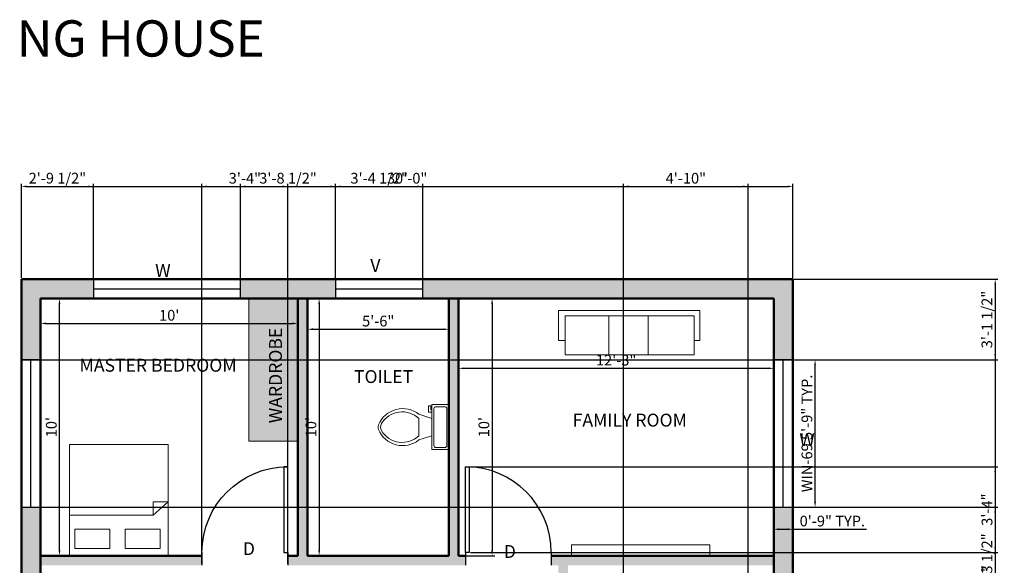
# Model space of a CAD drawing. Units: inches. Extents: x 2064 to 2999, y 1440 to 2089.
# Tile 7 of 7: x 2540 to 2999, y 1835 to 2089. Entities that reach past the tile are written whole.
import ezdxf

# ---------------------------------------------------------------- set-up
doc = ezdxf.new("R2010")
doc.units = ezdxf.units.IN
for name, color, linetype, lineweight in [('A-ANNO-DIMS', 2, 'Continuous', 18), ('A-ANNO-TEXT', 3, 'Continuous', 18), ('A-AREA-IDEN', 7, 'Continuous', 18), ('A-DOOR', 4, 'Continuous', 25), ('A-FLOR-FIXT', 9, 'Continuous', 18), ('A-FURN', 8, 'Continuous', 18), ('A-FURN-PATT', 252, 'Continuous', 13), ('A-GLAZ', 3, 'Continuous', 25), ('A-WALL', 7, 'Continuous', 50), ('A-WALL-PATT', 8, 'Continuous', 13)]:
    doc.layers.add(name, color=color, linetype=linetype, lineweight=lineweight)
doc.styles.get("Standard").update_dxf_attribs({"font": 'arial.ttf'})
doc.dimstyles.new('ISO-25', dxfattribs={"dimtxt": 5, "dimasz": 2.5, "dimexe": 1.25, "dimexo": 0.625, "dimtad": 1, "dimdec": 0, "dimlunit": 4, "dimtxsty": 'Standard', "dimcen": 2.5, "dimadec": 0, "dimazin": 0, "dimtfac": 1, "dimtdec": 0, "dimtmove": 0, "dimatfit": 3, "dimfxl": 1, "dimarcsym": 0})

# ---------------------------------------------------------------- blocks, each defined once
blk = doc.blocks.new('*U2')
for p, q in [((0, 0), (0, -6)), ((40, 0), (40, -6))]:
    blk.add_line(p, q)
blk.add_lwpolyline([(0, 0), (0, 40), (1.75, 40), (1.75, 0)], close=True)
blk.add_arc((0, 0), 40, 0, 90)
blk = doc.blocks.new('*U4')
for p, q in [((9.5, -6), (9.5, -2)), ((-10, -8.5), (-8, -8.5)), ((-10, -9.5), (-10, -8.5)), ((-8, -8.5), (-8, -8)), ((-7, -8), (-7, -9.5)), ((-4, -8), (-6, -14)), ((4, -8), (6, -14)), ((-7, -9.5), (-10, -9.5)), ((4, -14), (-4, -14))]:
    blk.add_line(p, q)
blk.add_lwpolyline([(10.5, -8), (10.5, 0), (-10.5, 0), (-10.5, -8)], close=True)
for points in [[(-9.5, -2), (-9.5, -6)], [(8.5, -1), (-8.5, -1)], [(-8.5, -7), (8.5, -7)]]:
    blk.add_lwpolyline(points)
for centre, radius, start, end in [((-8.62, -1.88), 0.884, 81.8699, 188.1301), ((8.62, -1.88), 0.884, 351.8699, 98.1301), ((-8.62, -6.12), 0.884, 171.8699, 278.1301), ((8.62, -6.12), 0.884, 261.8699, 8.1301), ((3.52, -21.58), 12.17, 141.4691, 247.9714), ((4.2, -21.82), 11.33, 136.3677, 238.9468), ((-3.52, -21.58), 12.17, 292.0284, 38.5307), ((-4.2, -21.82), 11.33, 301.053, 43.6321), ((0, -27.88), 4, 245.7318, 294.2682), ((0, -29), 4, 254.8605, 285.1395)]:
    blk.add_arc(centre, radius, start, end)
blk = doc.blocks.new('*D19')
at = {"layer": 'A-ANNO-DIMS', "color": 0, "lineweight": -2, "transparency": 16777216}
for p, q in [((2549.87, 1958.45), (2549.87, 1946.21)), ((2669.87, 1958.45), (2669.87, 1946.21)), ((2552.37, 1947.46), (2667.37, 1947.46))]:
    blk.add_line(p, q, dxfattribs=at)
at = {"layer": 'A-ANNO-DIMS', "color": 0, "transparency": 16777216}
for points in [[(2552.37, 1947.88), (2552.37, 1947.05), (2549.87, 1947.46)], [(2667.37, 1947.88), (2667.37, 1947.05), (2669.87, 1947.46)]]:
    blk.add_solid(points, dxfattribs=at)
at = {"layer": 'Defpoints', "color": 0, "transparency": 16777216}
for p in [(2549.87, 1959.07), (2669.87, 1959.07), (2669.87, 1947.46)]:
    blk.add_point(p, dxfattribs=at)
at = {"layer": 'A-ANNO-DIMS', "color": 0, "transparency": 16777216, "insert": (2609.87, 1950.64), "char_height": 5, "attachment_point": 5}
blk.add_mtext("10'", dxfattribs=at)
blk = doc.blocks.new('*D20')
at = {"layer": 'A-ANNO-DIMS', "color": 0, "lineweight": -2, "transparency": 16777216}
for p, q in [((2550.5, 1959.07), (2559.93, 1959.07)), ((2558.68, 1841.57), (2558.68, 1956.57)), ((2550.5, 1839.07), (2559.93, 1839.07))]:
    blk.add_line(p, q, dxfattribs=at)
at = {"layer": 'A-ANNO-DIMS', "color": 0, "transparency": 16777216}
for points in [[(2558.26, 1956.57), (2559.09, 1956.57), (2558.68, 1959.07)], [(2558.26, 1841.57), (2559.09, 1841.57), (2558.68, 1839.07)]]:
    blk.add_solid(points, dxfattribs=at)
at = {"layer": 'Defpoints', "color": 0, "transparency": 16777216}
for p in [(2549.87, 1959.07), (2558.68, 1959.07), (2549.87, 1839.07)]:
    blk.add_point(p, dxfattribs=at)
at = {"layer": 'A-ANNO-DIMS', "color": 0, "transparency": 16777216, "insert": (2555.5, 1899.07), "char_height": 5, "attachment_point": 5, "rotation": 90}
blk.add_mtext("10'", dxfattribs=at)
blk = doc.blocks.new('*D21')
at = {"layer": 'A-ANNO-DIMS', "color": 0, "lineweight": -2, "transparency": 16777216}
for p, q in [((2674.37, 1958.45), (2674.37, 1943.51)), ((2740.37, 1958.45), (2740.37, 1943.51)), ((2676.87, 1944.76), (2737.87, 1944.76))]:
    blk.add_line(p, q, dxfattribs=at)
at = {"layer": 'A-ANNO-DIMS', "color": 0, "transparency": 16777216}
for points in [[(2676.87, 1945.17), (2676.87, 1944.34), (2674.37, 1944.76)], [(2737.87, 1945.17), (2737.87, 1944.34), (2740.37, 1944.76)]]:
    blk.add_solid(points, dxfattribs=at)
at = {"layer": 'Defpoints', "color": 0, "transparency": 16777216}
for p in [(2674.37, 1959.07), (2740.37, 1959.07), (2740.37, 1944.76)]:
    blk.add_point(p, dxfattribs=at)
at = {"layer": 'A-ANNO-DIMS', "color": 0, "transparency": 16777216, "insert": (2707.37, 1947.93), "char_height": 5, "attachment_point": 5}
blk.add_mtext('5\'-6"', dxfattribs=at)
blk = doc.blocks.new('*D22')
at = {"layer": 'A-ANNO-DIMS', "color": 0, "lineweight": -2, "transparency": 16777216}
for p, q in [((2675, 1959.07), (2681.07, 1959.07)), ((2679.82, 1956.57), (2679.82, 1841.57)), ((2675, 1839.07), (2681.07, 1839.07))]:
    blk.add_line(p, q, dxfattribs=at)
at = {"layer": 'A-ANNO-DIMS', "color": 0, "transparency": 16777216}
for points in [[(2679.4, 1956.57), (2680.24, 1956.57), (2679.82, 1959.07)], [(2679.4, 1841.57), (2680.24, 1841.57), (2679.82, 1839.07)]]:
    blk.add_solid(points, dxfattribs=at)
at = {"layer": 'Defpoints', "color": 0, "transparency": 16777216}
for p in [(2674.37, 1959.07), (2674.37, 1839.07), (2679.82, 1839.07)]:
    blk.add_point(p, dxfattribs=at)
at = {"layer": 'A-ANNO-DIMS', "color": 0, "transparency": 16777216, "insert": (2676.64, 1899.07), "char_height": 5, "attachment_point": 5, "rotation": 90}
blk.add_mtext("10'", dxfattribs=at)
blk = doc.blocks.new('*D23')
at = {"layer": 'A-ANNO-DIMS', "color": 0, "lineweight": -2, "transparency": 16777216}
for p, q in [((2744.87, 1958.45), (2744.87, 1925.27)), ((2891.87, 1958.45), (2891.87, 1925.27)), ((2747.37, 1926.52), (2889.37, 1926.52))]:
    blk.add_line(p, q, dxfattribs=at)
at = {"layer": 'A-ANNO-DIMS', "color": 0, "transparency": 16777216}
for points in [[(2747.37, 1926.94), (2747.37, 1926.11), (2744.87, 1926.52)], [(2889.37, 1926.94), (2889.37, 1926.11), (2891.87, 1926.52)]]:
    blk.add_solid(points, dxfattribs=at)
at = {"layer": 'Defpoints', "color": 0, "transparency": 16777216}
for p in [(2744.87, 1959.07), (2891.87, 1959.07), (2891.87, 1926.52)]:
    blk.add_point(p, dxfattribs=at)
at = {"layer": 'A-ANNO-DIMS', "color": 0, "transparency": 16777216, "insert": (2818.37, 1929.7), "char_height": 5, "attachment_point": 5}
blk.add_mtext('12\'-3"', dxfattribs=at)
blk = doc.blocks.new('*D24')
at = {"layer": 'A-ANNO-DIMS', "color": 0, "lineweight": -2, "transparency": 16777216}
for p, q in [((2745.5, 1959.07), (2761.75, 1959.07)), ((2760.5, 1956.57), (2760.5, 1841.57)), ((2745.5, 1839.07), (2761.75, 1839.07))]:
    blk.add_line(p, q, dxfattribs=at)
at = {"layer": 'A-ANNO-DIMS', "color": 0, "transparency": 16777216}
for points in [[(2760.08, 1956.57), (2760.91, 1956.57), (2760.5, 1959.07)], [(2760.08, 1841.57), (2760.91, 1841.57), (2760.5, 1839.07)]]:
    blk.add_solid(points, dxfattribs=at)
at = {"layer": 'Defpoints', "color": 0, "transparency": 16777216}
for p in [(2744.87, 1959.07), (2744.87, 1839.07), (2760.5, 1839.07)]:
    blk.add_point(p, dxfattribs=at)
at = {"layer": 'A-ANNO-DIMS', "color": 0, "transparency": 16777216, "insert": (2757.32, 1899.07), "char_height": 5, "attachment_point": 5, "rotation": 90}
blk.add_mtext("10'", dxfattribs=at)
blk = doc.blocks.new('SOFA-3')
for p, q in [((0, 0), (0, 65.92)), ((0, 65.92), (14.01, 65.92)), ((14.01, 65.92), (14.01, 63.25)), ((20.61, 41.74), (2.39, 41.74)), ((20.61, 23.49), (2.39, 23.49)), ((14.01, 3.1), (14.01, 0)), ((14.01, 0), (0, 0))]:
    blk.add_line(p, q)
blk.add_lwpolyline([(2.39, 3.1), (20.61, 3.1), (20.61, 63.25), (2.39, 63.25)], close=True)
blk = doc.blocks.new('WIN-69')
blk.add_line((4.5, 0), (4.5, 68.8))
blk.add_lwpolyline([(0, 0), (9, 0), (9, 68.8), (0, 68.8)], close=True)
blk = doc.blocks.new('*D61')
at = {"layer": 'A-ANNO-DIMS', "color": 0, "lineweight": -2, "transparency": 16777216}
for p, q in [((2901.5, 1930.52), (2912.44, 1930.52)), ((2911.19, 1864.22), (2911.19, 1928.02)), ((2901.5, 1861.72), (2912.44, 1861.72))]:
    blk.add_line(p, q, dxfattribs=at)
at = {"layer": 'A-ANNO-DIMS', "color": 0, "transparency": 16777216}
for points in [[(2910.78, 1928.02), (2911.61, 1928.02), (2911.19, 1930.52)], [(2910.78, 1864.22), (2911.61, 1864.22), (2911.19, 1861.72)]]:
    blk.add_solid(points, dxfattribs=at)
at = {"layer": 'Defpoints', "color": 0, "transparency": 16777216}
for p in [(2900.87, 1930.52), (2911.19, 1930.52), (2900.87, 1861.72)]:
    blk.add_point(p, dxfattribs=at)
at = {"layer": 'A-ANNO-DIMS', "color": 0, "transparency": 16777216, "insert": (2908.02, 1896.12), "char_height": 5, "attachment_point": 5, "rotation": 90}
blk.add_mtext('WIN-69 5\'-9" TYP.', dxfattribs=at)
blk = doc.blocks.new('*D62')
at = {"layer": 'A-ANNO-DIMS', "color": 0, "lineweight": -2, "transparency": 16777216}
for p, q in [((2891.87, 1861.1), (2891.87, 1850.15)), ((2900.87, 1861.1), (2900.87, 1850.15)), ((2894.37, 1851.4), (2898.37, 1851.4)), ((2900.87, 1851.4), (2935.1, 1851.4))]:
    blk.add_line(p, q, dxfattribs=at)
at = {"layer": 'A-ANNO-DIMS', "color": 0, "transparency": 16777216}
for points in [[(2894.37, 1851.82), (2894.37, 1850.99), (2891.87, 1851.4)], [(2898.37, 1851.82), (2898.37, 1850.99), (2900.87, 1851.4)]]:
    blk.add_solid(points, dxfattribs=at)
at = {"layer": 'Defpoints', "color": 0, "transparency": 16777216}
for p in [(2891.87, 1861.72), (2900.87, 1861.72), (2900.87, 1851.4)]:
    blk.add_point(p, dxfattribs=at)
at = {"layer": 'A-ANNO-DIMS', "color": 0, "transparency": 16777216, "insert": (2919.24, 1854.58), "char_height": 5, "attachment_point": 5}
blk.add_mtext('0\'-9" TYP.', dxfattribs=at)
blk = doc.blocks.new('*D82')
at = {"layer": 'A-ANNO-DIMS', "color": 0, "lineweight": -2, "transparency": 16777216}
for p, q in [((2540.87, 1968.7), (2540.87, 2012.67)), ((2900.87, 1968.7), (2900.87, 2012.67)), ((2543.37, 2011.42), (2898.37, 2011.42))]:
    blk.add_line(p, q, dxfattribs=at)
at = {"layer": 'A-ANNO-DIMS', "color": 0, "transparency": 16777216}
for points in [[(2543.37, 2011.84), (2543.37, 2011), (2540.87, 2011.42)], [(2898.37, 2011.84), (2898.37, 2011), (2900.87, 2011.42)]]:
    blk.add_solid(points, dxfattribs=at)
at = {"layer": 'Defpoints', "color": 0, "transparency": 16777216}
for p in [(2900.87, 2011.42), (2540.87, 1968.07), (2900.87, 1968.07)]:
    blk.add_point(p, dxfattribs=at)
at = {"layer": 'A-ANNO-DIMS', "color": 0, "transparency": 16777216, "insert": (2720.87, 2014.6), "char_height": 5, "attachment_point": 5}
blk.add_mtext('30\'-0"', dxfattribs=at)
blk = doc.blocks.new('*D83')
at = {"layer": 'A-ANNO-DIMS', "color": 0, "lineweight": -2, "transparency": 16777216}
for p, q in [((2901.5, 1968.07), (2996.47, 1968.07)), ((2995.22, 1965.57), (2995.22, 1490.57)), ((2901.5, 1488.07), (2996.47, 1488.07))]:
    blk.add_line(p, q, dxfattribs=at)
at = {"layer": 'A-ANNO-DIMS', "color": 0, "transparency": 16777216}
for points in [[(2994.81, 1965.57), (2995.64, 1965.57), (2995.22, 1968.07)], [(2994.81, 1490.57), (2995.64, 1490.57), (2995.22, 1488.07)]]:
    blk.add_solid(points, dxfattribs=at)
at = {"layer": 'Defpoints', "color": 0, "transparency": 16777216}
for p in [(2900.87, 1968.07), (2900.87, 1488.07), (2995.22, 1488.07)]:
    blk.add_point(p, dxfattribs=at)
at = {"layer": 'A-ANNO-DIMS', "color": 0, "transparency": 16777216, "insert": (2992.05, 1728.07), "char_height": 5, "attachment_point": 5, "rotation": 90}
blk.add_mtext('40\'-0"', dxfattribs=at)
blk = doc.blocks.new('*D84')
at = {"layer": 'A-ANNO-DIMS', "color": 0, "lineweight": -2, "transparency": 16777216}
for p, q in [((2540.87, 1968.7), (2540.87, 2012.67)), ((2574.52, 1968.7), (2574.52, 2012.67)), ((2543.37, 2011.42), (2572.02, 2011.42))]:
    blk.add_line(p, q, dxfattribs=at)
at = {"layer": 'A-ANNO-DIMS', "color": 0, "transparency": 16777216}
for points in [[(2543.37, 2011.84), (2543.37, 2011), (2540.87, 2011.42)], [(2572.02, 2011.84), (2572.02, 2011), (2574.52, 2011.42)]]:
    blk.add_solid(points, dxfattribs=at)
at = {"layer": 'Defpoints', "color": 0, "transparency": 16777216}
for p in [(2574.52, 2011.42), (2540.87, 1968.07), (2574.52, 1968.07)]:
    blk.add_point(p, dxfattribs=at)
at = {"layer": 'A-ANNO-DIMS', "color": 0, "transparency": 16777216, "insert": (2557.7, 2014.63), "char_height": 5, "attachment_point": 5}
blk.add_mtext('2\'-9 1/2"', dxfattribs=at)
blk = doc.blocks.new('*D85')
at = {"layer": 'A-ANNO-DIMS', "color": 0, "lineweight": -2, "transparency": 16777216}
for p, q in [((2643.06, 1968.7), (2643.06, 2012.67)), ((2687.51, 1968.7), (2687.51, 2012.67)), ((2645.56, 2011.42), (2685.01, 2011.42))]:
    blk.add_line(p, q, dxfattribs=at)
at = {"layer": 'A-ANNO-DIMS', "color": 0, "transparency": 16777216}
for points in [[(2645.56, 2011.84), (2645.56, 2011), (2643.06, 2011.42)], [(2685.01, 2011.84), (2685.01, 2011), (2687.51, 2011.42)]]:
    blk.add_solid(points, dxfattribs=at)
at = {"layer": 'Defpoints', "color": 0, "transparency": 16777216}
for p in [(2687.51, 2011.42), (2643.06, 1968.07), (2687.51, 1968.07)]:
    blk.add_point(p, dxfattribs=at)
at = {"layer": 'A-ANNO-DIMS', "color": 0, "transparency": 16777216, "insert": (2665.29, 2014.63), "char_height": 5, "attachment_point": 5}
blk.add_mtext('3\'-8 1/2"', dxfattribs=at)
blk = doc.blocks.new('*D86')
at = {"layer": 'A-ANNO-DIMS', "color": 0, "lineweight": -2, "transparency": 16777216}
for p, q in [((2687.51, 1968.7), (2687.51, 2012.67)), ((2728.11, 1968.7), (2728.11, 2012.67)), ((2690.01, 2011.42), (2725.61, 2011.42))]:
    blk.add_line(p, q, dxfattribs=at)
at = {"layer": 'A-ANNO-DIMS', "color": 0, "transparency": 16777216}
for points in [[(2690.01, 2011.84), (2690.01, 2011), (2687.51, 2011.42)], [(2725.61, 2011.84), (2725.61, 2011), (2728.11, 2011.42)]]:
    blk.add_solid(points, dxfattribs=at)
at = {"layer": 'Defpoints', "color": 0, "transparency": 16777216}
for p in [(2728.11, 2011.42), (2687.51, 1968.07), (2728.11, 1968.07)]:
    blk.add_point(p, dxfattribs=at)
at = {"layer": 'A-ANNO-DIMS', "color": 0, "transparency": 16777216, "insert": (2707.81, 2014.63), "char_height": 5, "attachment_point": 5}
blk.add_mtext('3\'-4 1/2"', dxfattribs=at)
blk = doc.blocks.new('*D87')
at = {"layer": 'A-ANNO-DIMS', "color": 0, "lineweight": -2, "transparency": 16777216}
for p, q in [((2901.5, 1968.07), (2996.47, 1968.07)), ((2995.22, 1965.57), (2995.22, 1933.02)), ((2901.5, 1930.52), (2996.47, 1930.52))]:
    blk.add_line(p, q, dxfattribs=at)
at = {"layer": 'A-ANNO-DIMS', "color": 0, "transparency": 16777216}
for points in [[(2994.81, 1965.57), (2995.64, 1965.57), (2995.22, 1968.07)], [(2994.81, 1933.02), (2995.64, 1933.02), (2995.22, 1930.52)]]:
    blk.add_solid(points, dxfattribs=at)
at = {"layer": 'Defpoints', "color": 0, "transparency": 16777216}
for p in [(2900.87, 1968.07), (2900.87, 1930.52), (2995.22, 1930.52)]:
    blk.add_point(p, dxfattribs=at)
at = {"layer": 'A-ANNO-DIMS', "color": 0, "transparency": 16777216, "insert": (2992.01, 1949.3), "char_height": 5, "attachment_point": 5, "rotation": 90}
blk.add_mtext('3\'-1 1/2"', dxfattribs=at)
blk = doc.blocks.new('*D88')
at = {"layer": 'A-ANNO-DIMS', "color": 0, "lineweight": -2, "transparency": 16777216}
for p, q in [((2901.5, 1861.72), (2996.47, 1861.72)), ((2995.22, 1859.22), (2995.22, 1812.91)), ((2901.5, 1810.41), (2996.47, 1810.41))]:
    blk.add_line(p, q, dxfattribs=at)
at = {"layer": 'A-ANNO-DIMS', "color": 0, "transparency": 16777216}
for points in [[(2994.81, 1859.22), (2995.64, 1859.22), (2995.22, 1861.72)], [(2994.81, 1812.91), (2995.64, 1812.91), (2995.22, 1810.41)]]:
    blk.add_solid(points, dxfattribs=at)
at = {"layer": 'Defpoints', "color": 0, "transparency": 16777216}
for p in [(2900.87, 1861.72), (2900.87, 1810.41), (2995.22, 1810.41)]:
    blk.add_point(p, dxfattribs=at)
at = {"layer": 'A-ANNO-DIMS', "color": 0, "transparency": 16777216, "insert": (2992.01, 1836.07), "char_height": 5, "attachment_point": 5, "rotation": 90}
blk.add_mtext('4\'-3 1/2"', dxfattribs=at)
blk = doc.blocks.new('*D91')
at = {"layer": 'A-ANNO-DIMS', "color": 0, "lineweight": -2, "transparency": 16777216}
for p, q in [((2541.5, 1968.07), (2996.47, 1968.07)), ((2995.22, 1965.57), (2995.22, 1933.02)), ((2541.5, 1930.52), (2996.47, 1930.52))]:
    blk.add_line(p, q, dxfattribs=at)
at = {"layer": 'A-ANNO-DIMS', "color": 0, "transparency": 16777216}
for points in [[(2994.81, 1965.57), (2995.64, 1965.57), (2995.22, 1968.07)], [(2994.81, 1933.02), (2995.64, 1933.02), (2995.22, 1930.52)]]:
    blk.add_solid(points, dxfattribs=at)
at = {"layer": 'Defpoints', "color": 0, "transparency": 16777216}
for p in [(2540.87, 1968.07), (2540.87, 1930.52), (2995.22, 1930.52)]:
    blk.add_point(p, dxfattribs=at)
at = {"layer": 'A-ANNO-DIMS', "color": 0, "transparency": 16777216, "insert": (2992.01, 1949.3), "char_height": 5, "attachment_point": 5, "rotation": 90}
blk.add_mtext('3\'-1 1/2"', dxfattribs=at)
blk = doc.blocks.new('*D92')
at = {"layer": 'A-ANNO-DIMS', "color": 0, "lineweight": -2, "transparency": 16777216}
for p, q in [((2541.5, 1861.72), (2996.47, 1861.72)), ((2995.22, 1859.22), (2995.22, 1795.07)), ((2541.5, 1792.57), (2996.47, 1792.57))]:
    blk.add_line(p, q, dxfattribs=at)
at = {"layer": 'A-ANNO-DIMS', "color": 0, "transparency": 16777216}
for points in [[(2994.81, 1859.22), (2995.64, 1859.22), (2995.22, 1861.72)], [(2994.81, 1795.07), (2995.64, 1795.07), (2995.22, 1792.57)]]:
    blk.add_solid(points, dxfattribs=at)
at = {"layer": 'Defpoints', "color": 0, "transparency": 16777216}
for p in [(2540.87, 1861.72), (2540.87, 1792.57), (2995.22, 1792.57)]:
    blk.add_point(p, dxfattribs=at)
at = {"layer": 'A-ANNO-DIMS', "color": 0, "transparency": 16777216, "insert": (2992.05, 1827.15), "char_height": 5, "attachment_point": 5, "rotation": 90}
blk.add_mtext('5\'-9"', dxfattribs=at)
blk = doc.blocks.new('*D104')
at = {"layer": 'A-ANNO-DIMS', "color": 0, "lineweight": -2, "transparency": 16777216}
for p, q in [((2821.8, 1758.7), (2821.8, 2012.67)), ((2879.97, 1758.7), (2879.97, 2012.67)), ((2824.3, 2011.42), (2877.47, 2011.42))]:
    blk.add_line(p, q, dxfattribs=at)
at = {"layer": 'A-ANNO-DIMS', "color": 0, "transparency": 16777216}
for points in [[(2824.3, 2011.84), (2824.3, 2011), (2821.8, 2011.42)], [(2877.47, 2011.84), (2877.47, 2011), (2879.97, 2011.42)]]:
    blk.add_solid(points, dxfattribs=at)
at = {"layer": 'Defpoints', "color": 0, "transparency": 16777216}
for p in [(2879.97, 2011.42), (2821.8, 1758.07), (2879.97, 1758.07)]:
    blk.add_point(p, dxfattribs=at)
at = {"layer": 'A-ANNO-DIMS', "color": 0, "transparency": 16777216, "insert": (2850.89, 2014.6), "char_height": 5, "attachment_point": 5}
blk.add_mtext('4\'-10"', dxfattribs=at)
blk = doc.blocks.new('*D115')
at = {"layer": 'A-ANNO-DIMS', "color": 0, "lineweight": -2, "transparency": 16777216}
for p, q in [((2625.15, 1835.2), (2625.15, 2012.67)), ((2665.15, 1835.2), (2665.15, 2012.67)), ((2627.65, 2011.42), (2662.65, 2011.42))]:
    blk.add_line(p, q, dxfattribs=at)
at = {"layer": 'A-ANNO-DIMS', "color": 0, "transparency": 16777216}
for points in [[(2627.65, 2011.84), (2627.65, 2011), (2625.15, 2011.42)], [(2662.65, 2011.84), (2662.65, 2011), (2665.15, 2011.42)]]:
    blk.add_solid(points, dxfattribs=at)
at = {"layer": 'Defpoints', "color": 0, "transparency": 16777216}
for p in [(2665.15, 2011.42), (2625.15, 1834.57), (2665.15, 1834.57)]:
    blk.add_point(p, dxfattribs=at)
at = {"layer": 'A-ANNO-DIMS', "color": 0, "transparency": 16777216, "insert": (2645.15, 2014.6), "char_height": 5, "attachment_point": 5}
blk.add_mtext('3\'-4"', dxfattribs=at)
blk = doc.blocks.new('*D116')
at = {"layer": 'A-ANNO-DIMS', "color": 0, "lineweight": -2, "transparency": 16777216}
for p, q in [((2750.49, 1880.57), (2996.47, 1880.57)), ((2995.22, 1878.07), (2995.22, 1843.07)), ((2750.49, 1840.57), (2996.47, 1840.57))]:
    blk.add_line(p, q, dxfattribs=at)
at = {"layer": 'A-ANNO-DIMS', "color": 0, "transparency": 16777216}
for points in [[(2994.81, 1878.07), (2995.64, 1878.07), (2995.22, 1880.57)], [(2994.81, 1843.07), (2995.64, 1843.07), (2995.22, 1840.57)]]:
    blk.add_solid(points, dxfattribs=at)
at = {"layer": 'Defpoints', "color": 0, "transparency": 16777216}
for p in [(2749.86, 1880.57), (2749.86, 1840.57), (2995.22, 1840.57)]:
    blk.add_point(p, dxfattribs=at)
at = {"layer": 'A-ANNO-DIMS', "color": 0, "transparency": 16777216, "insert": (2992.05, 1860.57), "char_height": 5, "attachment_point": 5, "rotation": 90}
blk.add_mtext('3\'-4"', dxfattribs=at)

msp = doc.modelspace()

# ---------------------------------------------------------------- hatches: boundary and pattern name
at = {"layer": 'A-FURN-PATT'}
h = msp.add_hatch(color=256, dxfattribs=at)
h.dxf.hatch_style = 1
h.paths.add_polyline_path([(2211.98, 1959.07), (2126.82, 1959.07), (2126.82, 1938.57), (2211.98, 1938.57)])
h.paths.add_polyline_path([(2669.87, 1959.07), (2646.96, 1959.07), (2646.96, 1892.49), (2669.87, 1892.49)])
h.paths.add_polyline_path([(2468.82, 1668.53), (2348.82, 1668.53), (2348.82, 1638.07), (2468.82, 1638.07)])
h.paths.add_polyline_path([(2891.87, 1667.99), (2780.13, 1667.99), (2780.13, 1638.07), (2891.87, 1638.07)])
h.paths.add_polyline_path([(2854.27, 1658.75), (2854.27, 1650.97), (2859.31, 1650.97), (2859.31, 1658.75), (2862.16, 1658.75), (2862.16, 1650.97), (2867.47, 1650.97), (2867.47, 1658.75), (2870.33, 1658.75), (2870.33, 1650.97), (2879.45, 1650.97), (2879.45, 1658.75), (2882.31, 1658.75), (2882.31, 1643.24), (2879.45, 1643.24), (2879.45, 1650.97), (2870.33, 1650.97), (2870.33, 1643.24), (2867.47, 1643.24), (2867.47, 1650.97), (2862.16, 1650.97), (2862.16, 1643.24), (2859.31, 1643.24), (2859.31, 1650.97), (2854.27, 1650.97), (2854.27, 1643.24), (2851.41, 1643.24), (2851.41, 1650.97), (2845.97, 1650.97), (2845.97, 1643.24), (2843.11, 1643.24), (2843.11, 1650.97), (2839.98, 1650.97), (2839.98, 1643.24), (2837.12, 1643.24), (2837.12, 1650.97), (2831.27, 1650.97), (2831.27, 1643.24), (2828.41, 1643.24), (2828.41, 1650.97), (2823.78, 1650.97), (2823.78, 1643.24), (2820.92, 1643.24), (2820.92, 1650.97), (2816.56, 1650.97), (2816.56, 1641.66), (2813.71, 1641.66), (2813.71, 1650.97), (2808.81, 1650.97), (2808.81, 1641.66), (2805.95, 1641.66), (2805.95, 1650.97), (2801.73, 1650.97), (2801.73, 1641.66), (2798.87, 1641.66), (2798.87, 1650.97), (2794.92, 1650.97), (2794.92, 1643.24), (2792.06, 1643.24), (2792.06, 1658.75), (2794.92, 1658.75), (2794.92, 1650.97), (2798.87, 1650.97), (2798.87, 1657.16), (2801.73, 1657.16), (2801.73, 1650.97), (2805.95, 1650.97), (2805.95, 1657.16), (2808.81, 1657.16), (2808.81, 1650.97), (2813.71, 1650.97), (2813.71, 1657.16), (2816.56, 1657.16), (2816.56, 1650.97), (2820.92, 1650.97), (2820.92, 1658.75), (2823.78, 1658.75), (2823.78, 1650.97), (2828.41, 1650.97), (2828.41, 1658.75), (2831.27, 1658.75), (2831.27, 1650.97), (2837.12, 1650.97), (2837.12, 1658.75), (2839.98, 1658.75), (2839.98, 1650.97), (2843.11, 1650.97), (2843.11, 1658.75), (2845.97, 1658.75), (2845.97, 1650.97), (2851.41, 1650.97), (2851.41, 1658.75)], flags=16)
h.paths.add_polyline_path([(2665.84, 1899.31), (2665.84, 1951.8), (2653.45, 1951.8), (2653.45, 1899.31)], flags=24)
h.paths.add_polyline_path([(2565.91, 1921.55), (2649.69, 1921.55), (2649.69, 1933.95), (2565.91, 1933.95)], flags=9)
h.paths.add_polyline_path([(2402.8, 1649), (2414.4, 1649), (2414.4, 1659.3), (2402.8, 1659.3)], flags=24)
at = {"layer": 'A-WALL-PATT'}
h = msp.add_hatch(color=256, dxfattribs=at)
h.dxf.hatch_style = 1
h.paths.add_polyline_path([(2574.52, 1968.07), (2540.87, 1968.07), (2540.87, 1930.52), (2549.87, 1930.52), (2549.87, 1959.07), (2574.52, 1959.07)])
h.paths.add_polyline_path([(2687.51, 1968.07), (2643.06, 1968.07), (2643.06, 1959.07), (2669.87, 1959.07), (2687.51, 1959.07)])
h.paths.add_polyline_path([(2900.87, 1968.07), (2728.11, 1968.07), (2728.11, 1959.07), (2740.37, 1959.07), (2891.87, 1959.07), (2891.87, 1930.52), (2900.87, 1930.52)])
h.paths.add_polyline_path([(2744.87, 1959.07), (2740.37, 1959.07), (2740.37, 1839.07), (2674.37, 1839.07), (2674.37, 1959.07), (2669.87, 1959.07), (2669.87, 1892.49), (2669.87, 1839.07), (2665.15, 1839.07), (2665.15, 1834.57), (2674.37, 1834.57), (2744.87, 1834.57), (2748.11, 1834.57), (2748.11, 1839.07), (2744.87, 1839.07)])
h.paths.add_polyline_path([(2549.87, 1834.57), (2549.87, 1861.72), (2540.87, 1861.72), (2540.87, 1792.57), (2549.87, 1792.57)])
h.paths.add_polyline_path([(2625.15, 1839.07), (2549.87, 1839.07), (2549.87, 1834.57), (2625.15, 1834.57)])
h.paths.add_polyline_path([(2900.87, 1861.72), (2891.87, 1861.72), (2891.87, 1810.41), (2900.87, 1810.41)])
h.paths.add_polyline_path([(2891.87, 1839.07), (2788.11, 1839.07), (2788.11, 1834.57), (2891.87, 1834.57)])
h.paths.add_polyline_path([(2549.87, 1745.09), (2540.87, 1745.09), (2540.87, 1697.07), (2549.87, 1697.07)])
h.paths.add_polyline_path([(2549.87, 1619.25), (2540.87, 1619.25), (2540.87, 1612.26), (2549.87, 1612.26)], flags=17)
h.paths.add_polyline_path([(2549.87, 1516.02), (2540.87, 1516.02), (2540.87, 1488.07), (2900.87, 1488.07), (2900.87, 1682.51), (2891.87, 1682.51), (2891.87, 1497.07), (2549.87, 1497.07)])
h.paths.add_polyline_path([(2771.87, 1575.08), (2767.37, 1575.08), (2767.37, 1497.07), (2771.87, 1497.07)], flags=17)
h.paths.add_polyline_path([(2771.87, 1708.85), (2767.37, 1708.85), (2767.37, 1633.57), (2771.87, 1633.57), (2771.87, 1638.07)])
h.paths.add_polyline_path([(2891.87, 1638.07), (2780.13, 1638.07), (2771.87, 1638.07), (2771.87, 1633.57), (2891.87, 1633.57)], flags=17)
h.paths.add_polyline_path([(2771.87, 1633.57), (2767.37, 1633.57), (2767.37, 1615.08), (2771.87, 1615.08)], flags=17)
h.paths.add_polyline_path([(2900.87, 1784.26), (2891.87, 1784.26), (2891.87, 1751.31), (2900.87, 1751.31)])
h.paths.add_polyline_path([(2795.87, 1834.57), (2791.37, 1834.57), (2791.37, 1830.13), (2795.87, 1830.13)])
h.paths.add_polyline_path([(2805.14, 1771.92), (2830.56, 1771.92), (2830.56, 1784.32), (2805.14, 1784.32)], flags=9)
h.paths.add_polyline_path([(2805.18, 1686.98), (2865.14, 1686.98), (2865.14, 1699.38), (2805.18, 1699.38)], flags=9)
h.paths.add_polyline_path([(2801, 1552.43), (2850.22, 1552.43), (2850.22, 1564.83), (2801, 1564.83)], flags=25)
h.paths.add_polyline_path([(2645.3, 1586.75), (2705.73, 1586.75), (2705.73, 1599.14), (2645.3, 1599.14)], flags=25)
h.paths.add_polyline_path([(2670.49, 1736.4), (2713.67, 1736.4), (2713.67, 1748.79), (2670.49, 1748.79)], flags=9)
h.paths.add_polyline_path([(2795.9, 1895.95), (2857.73, 1895.95), (2857.73, 1908.34), (2795.9, 1908.34)], flags=9)
h.paths.add_polyline_path([(2565.91, 1921.55), (2649.69, 1921.55), (2649.69, 1933.95), (2565.91, 1933.95)], flags=9)

# ---------------------------------------------------------------- linework, layer by layer
at = {"layer": 'A-FURN'}
for p, q in [((2602.33, 1858.02), (2602.33, 1864.23)), ((2602.33, 1864.23), (2609.36, 1864.23)), ((2609.36, 1864.23), (2602.33, 1858.02)), ((2563.4, 1858.02), (2602.33, 1858.02))]:
    msp.add_line(p, q, dxfattribs=at)
for points in [[(2669.87, 1959.07), (2646.96, 1959.07), (2646.96, 1892.49), (2669.87, 1892.49)], [(2563.4, 1839.07), (2609.36, 1839.07), (2609.36, 1891.01), (2563.4, 1891.01)], [(2565.89, 1842.42), (2582.11, 1842.42), (2582.11, 1851.45), (2565.89, 1851.45)], [(2589.38, 1842.42), (2605.6, 1842.42), (2605.6, 1851.45), (2589.38, 1851.45)], [(2797.55, 1839.07), (2862.05, 1839.07), (2862.05, 1844.06), (2797.55, 1844.06)]]:
    msp.add_lwpolyline(points, close=True, dxfattribs=at)
at = {"layer": 'A-GLAZ'}
for p, q in [((2574.52, 1963.57), (2643.06, 1963.57)), ((2687.51, 1963.57), (2728.11, 1963.57))]:
    msp.add_line(p, q, dxfattribs=at)
for points in [[(2574.52, 1959.07), (2643.06, 1959.07), (2643.06, 1968.07), (2574.52, 1968.07)], [(2687.51, 1959.07), (2728.11, 1959.07), (2728.11, 1968.07), (2687.51, 1968.07)]]:
    msp.add_lwpolyline(points, close=True, dxfattribs=at)
at = {"layer": 'A-WALL'}
for p, q in [((2540.87, 1968.07), (2900.87, 1968.07)), ((2540.87, 1488.07), (2540.87, 1968.07)), ((2900.87, 1968.07), (2900.87, 1488.07)), ((2549.87, 1959.07), (2891.87, 1959.07)), ((2549.87, 1497.07), (2549.87, 1959.07)), ((2549.87, 1959.07), (2669.87, 1959.07)), ((2669.87, 1959.07), (2669.87, 1839.07)), ((2674.37, 1959.07), (2674.37, 1839.07)), ((2674.37, 1959.07), (2740.37, 1959.07)), ((2740.37, 1959.07), (2740.37, 1839.07)), ((2744.87, 1959.07), (2744.87, 1839.07)), ((2891.87, 1959.07), (2891.87, 1497.07)), ((2625.15, 1839.07), (2549.87, 1839.07)), ((2669.87, 1839.07), (2665.15, 1839.07)), ((2740.37, 1839.07), (2674.37, 1839.07)), ((2744.87, 1839.07), (2748.11, 1839.07)), ((2788.11, 1839.07), (2891.87, 1839.07))]:
    msp.add_line(p, q, dxfattribs=at)

# ---------------------------------------------------------------- block references
at = {"layer": 'A-DOOR', "xscale": -1}
msp.add_blockref('*U2', (2665.15, 1840.57), dxfattribs=at)
at = {"layer": 'A-DOOR'}
msp.add_blockref('*U2', (2748.11, 1840.57), dxfattribs=at)
at = {"layer": 'A-FLOR-FIXT', "rotation": 270}
msp.add_blockref('*U4', (2740.37, 1899.07), dxfattribs=at)
at = {"layer": 'A-FURN', "rotation": 269.9999999999988}
msp.add_blockref('SOFA-3', (2791.5, 1953.45), dxfattribs=at)
at = {"layer": 'A-GLAZ'}
for p in [(2540.87, 1861.72), (2891.87, 1861.72)]:
    msp.add_blockref('WIN-69', p, dxfattribs=at)

# ---------------------------------------------------------------- texts
at = {"layer": 'A-ANNO-TEXT', "attachment_point": 1}
for s, width, gutter_width, heights, insert, char_height in [('EAST FACING HOUSE', 429.6774, 84.65, [17.52], (2430, 2088.96), 16.9292), ('V', 152.6727, 30.08, [0], (2703.68, 1977.54), 6.02), ('W', 152.6727, 30.08, [0], (2603.32, 1975.23), 6.02), ('W', 152.6727, 30.08, [0], (2903.83, 1896.23), 6.02), ('D', 152.6727, 30.08, [0], (2644.22, 1845.35), 6.02), ('D', 152.6727, 30.08, [0], (2765.96, 1844.03), 6.02)]:
    msp.add_mtext_dynamic_manual_height_columns(s, width=width, gutter_width=gutter_width, heights=heights, dxfattribs=dict(at, insert=insert, char_height=char_height))
at = {"layer": 'A-AREA-IDEN', "insert": (2656.44, 1900.91), "char_height": 6.015, "attachment_point": 1, "rotation": 90}
msp.add_mtext_dynamic_manual_height_columns('WARDROBE', width=152.6727, gutter_width=30.08, heights=[0], dxfattribs=at)
at = {"layer": 'A-AREA-IDEN', "attachment_point": 1}
for s, insert, char_height in [('MASTER BEDROOM', (2568.04, 1930.96), 6.0153), ('TOILET', (2696.06, 1925.68), 6.015), ('FAMILY ROOM', (2798.09, 1905.35), 6.0153)]:
    msp.add_mtext_dynamic_manual_height_columns(s, width=152.6727, gutter_width=30.08, heights=[0], dxfattribs=dict(at, insert=insert, char_height=char_height))

# ---------------------------------------------------------------- dimensions: what is measured, and where the dimension line sits
at = {"layer": 'A-ANNO-DIMS'}
for base, p1, p2, override, picture, middle in [((2574.5162, 2011.4209), (2540.8749, 1968.0709), (2574.5162, 1968.0709), {"dimdec": 1, "dimlfac": 1, "dimrnd": 0, "dimzin": 1, "dimdsep": 46, "dimlunit": 4, "dimfrac": 2}, '*D84', (2557.6956, 2014.6312)), ((2687.5143, 2011.4209), (2643.0615, 1968.0709), (2687.5143, 1968.0709), {"dimdec": 1, "dimlfac": 1, "dimrnd": 0, "dimzin": 1, "dimdsep": 46, "dimlunit": 4, "dimfrac": 2}, '*D85', (2665.2879, 2014.6329)), ((2728.11, 2011.42), (2687.51, 1968.07), (2728.11, 1968.07), {"dimdec": 1, "dimlfac": 1, "dimrnd": 0, "dimzin": 1, "dimdsep": 46, "dimlunit": 4, "dimfrac": 2}, '*D86', (2707.81, 2014.63)), ((2900.87, 2011.42), (2540.87, 1968.07), (2900.87, 1968.07), {"dimdec": 1, "dimlfac": 1, "dimrnd": 0, "dimzin": 1, "dimdsep": 46, "dimlunit": 4, "dimfrac": 2}, '*D82', (2720.87, 2014.6)), ((2665.15, 2011.42), (2625.15, 1834.57), (2665.15, 1834.57), {"dimdec": 1, "dimlfac": 1, "dimrnd": 0, "dimzin": 1, "dimdsep": 46, "dimlunit": 4, "dimfrac": 2}, '*D115', (2645.15, 2014.6)), ((2879.97, 2011.42), (2821.8, 1758.07), (2879.97, 1758.07), {"dimdec": 1, "dimlfac": 1, "dimrnd": 0, "dimzin": 1, "dimdsep": 46, "dimlunit": 4, "dimfrac": 2}, '*D104', (2850.89, 2014.6)), ((2669.87, 1947.46), (2549.87, 1959.07), (2669.87, 1959.07), {"dimclrd": 0, "dimclre": 0, "dimclrt": 0}, '*D19', (2609.87, 1950.64)), ((2740.37, 1944.76), (2674.37, 1959.07), (2740.37, 1959.07), {"dimclrd": 0, "dimclre": 0, "dimclrt": 0}, '*D21', (2707.37, 1947.93)), ((2891.87, 1926.52), (2744.87, 1959.07), (2891.87, 1959.07), {"dimclrd": 0, "dimclre": 0, "dimclrt": 0}, '*D23', (2818.37, 1929.7))]:
    dim = msp.add_linear_dim(base=base, p1=p1, p2=p2, dimstyle='ISO-25', override=override, dxfattribs=at)
    dim.commit()
    dim.dimension.update_dxf_attribs({"geometry": picture, "text_midpoint": middle})
for base, p1, p2, override, picture, middle in [((2995.2249, 1930.5223), (2540.8749, 1968.0709), (2540.8749, 1930.5223), {"dimdec": 1, "dimlfac": 1, "dimrnd": 0, "dimzin": 1, "dimdsep": 46, "dimlunit": 4, "dimfrac": 2}, '*D91', (2992.013, 1949.2966)), ((2995.22, 1488.07), (2900.87, 1968.07), (2900.87, 1488.07), {"dimdec": 1, "dimlfac": 1, "dimrnd": 0, "dimzin": 1, "dimdsep": 46, "dimlunit": 4, "dimfrac": 2}, '*D83', (2992.05, 1728.07)), ((2995.2249, 1930.5223), (2900.8749, 1968.0709), (2900.8749, 1930.5223), {"dimdec": 1, "dimlfac": 1, "dimrnd": 0, "dimzin": 1, "dimdsep": 46, "dimlunit": 4, "dimfrac": 2}, '*D87', (2992.013, 1949.2966)), ((2558.68, 1959.07), (2549.87, 1839.07), (2549.87, 1959.07), {"dimclrd": 0, "dimclre": 0, "dimclrt": 0}, '*D20', (2555.5, 1899.07)), ((2679.82, 1839.07), (2674.37, 1959.07), (2674.37, 1839.07), {"dimclrd": 0, "dimclre": 0, "dimclrt": 0}, '*D22', (2676.64, 1899.07)), ((2760.5, 1839.07), (2744.87, 1959.07), (2744.87, 1839.07), {"dimclrd": 0, "dimclre": 0, "dimclrt": 0}, '*D24', (2757.32, 1899.07)), ((2995.22, 1840.57), (2749.86, 1880.57), (2749.86, 1840.57), {"dimdec": 1, "dimlfac": 1, "dimrnd": 0, "dimzin": 1, "dimdsep": 46, "dimlunit": 4, "dimfrac": 2}, '*D116', (2992.05, 1860.57)), ((2995.2249, 1792.5709), (2540.8749, 1861.7244), (2540.8749, 1792.5709), {"dimdec": 1, "dimlfac": 1, "dimrnd": 0, "dimzin": 1, "dimdsep": 46, "dimlunit": 4, "dimfrac": 2}, '*D92', (2992.0471, 1827.1477)), ((2995.22, 1810.41), (2900.87, 1861.72), (2900.87, 1810.41), {"dimdec": 1, "dimlfac": 1, "dimrnd": 0, "dimzin": 1, "dimdsep": 46, "dimlunit": 4, "dimfrac": 2}, '*D88', (2992.01, 1836.07))]:
    dim = msp.add_linear_dim(base=base, p1=p1, p2=p2, angle=90, dimstyle='ISO-25', override=override, dxfattribs=at)
    dim.commit()
    dim.dimension.update_dxf_attribs({"geometry": picture, "text_midpoint": middle})
dim = msp.add_linear_dim(base=(2911.19, 1930.52), p1=(2900.87, 1861.72), p2=(2900.87, 1930.52), angle=90, text='WIN-69 <> TYP.', dimstyle='ISO-25', override={"dimdec": 1, "dimrnd": 0, "dimzin": 1, "dimlunit": 4, "dimfrac": 2}, dxfattribs=at)
dim.commit()
dim.dimension.update_dxf_attribs({"geometry": '*D61', "text_midpoint": (2908.02, 1896.12)})
dim = msp.add_linear_dim(base=(2900.87, 1851.4), p1=(2891.87, 1861.72), p2=(2900.87, 1861.72), text='<> TYP.', dimstyle='ISO-25', override={"dimdec": 1, "dimrnd": 0, "dimzin": 1, "dimlunit": 4, "dimfrac": 2}, dxfattribs=at)
dim.commit()
dim.dimension.update_dxf_attribs({"geometry": '*D62', "text_midpoint": (2919.24, 1854.58)})

doc.saveas('drawing.dxf')
